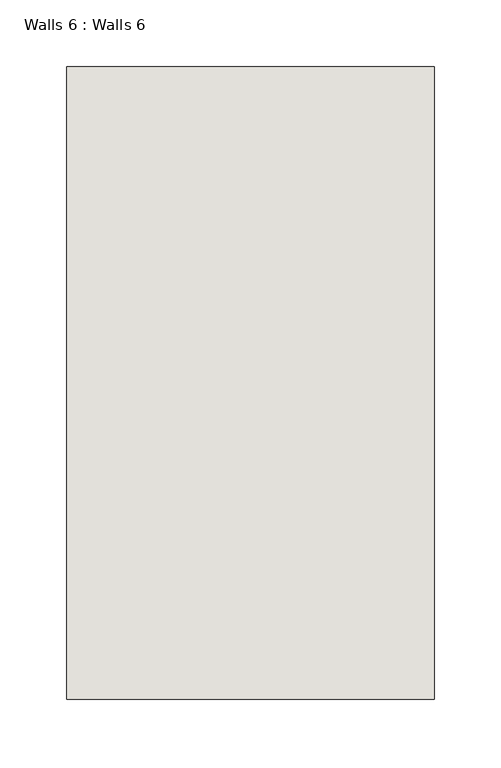
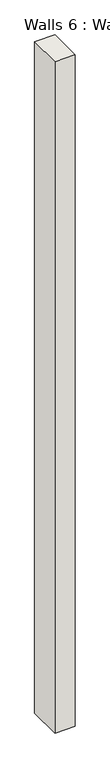
"""IFC4 building model written with IfcOpenShell, lengths in millimetres: wall geometry, Walls 6 : Walls 6."""

from ifc_helpers import new_model, si_unit, frame, origin, place, context, project, spatial, polyline, outline, extrude, source, transform, mapped, element, save


def walls_6_walls_6_1b60e08d(model_context):
    return source(origin(), model_context, "Body", "SweptSolid", [
        extrude(outline(polyline([(7778.3159626, -1369.3115858), (7502.1864593, -1369.3115858), (7502.1864593, -893.9851555), (7778.3159626, -893.9851555), (7778.3159626, -1369.3115858)])), frame((0.0, 0.0, 3048.0), z_axis=(0.0, 0.0, 1.0), x_axis=(1.0, 0.0, 0.0)), (0.0, 0.0, 1.0), 9642.9432281),
    ])


if __name__ == "__main__":
    model = new_model("IFC4")
    model_context = context("Model", 3, world=origin())
    ifc_project = project(units=[si_unit("LENGTHUNIT", "METRE", prefix="MILLI")], contexts=[model_context])
    site = spatial("IfcSite", under=ifc_project)
    building = spatial("IfcBuilding", under=site)
    placement = place(None, origin())
    walls_6_walls_6_shape = walls_6_walls_6_1b60e08d(model_context)
    element("IfcWall", 1, ObjectType="Walls 6 : Walls 6", at=placement, inside=building, context=model_context, shape_type="MappedRepresentation", body=[
        mapped(walls_6_walls_6_shape, transform((0.0, 0.0, 0.0), x_axis=(1.0, 0.0, 0.0), y_axis=(0.0, 1.0, 0.0), z_axis=(0.0, 0.0, 1.0))),
    ])
    save(model, "model.ifc")

# Revit data of these elements
# Element 1 (IfcWall, "Walls 6 : Walls 6")
#   Materials on its faces: "Default Wall"
# Materials
#   "Default Wall": colour RGB 80 80 80, transparency 0
